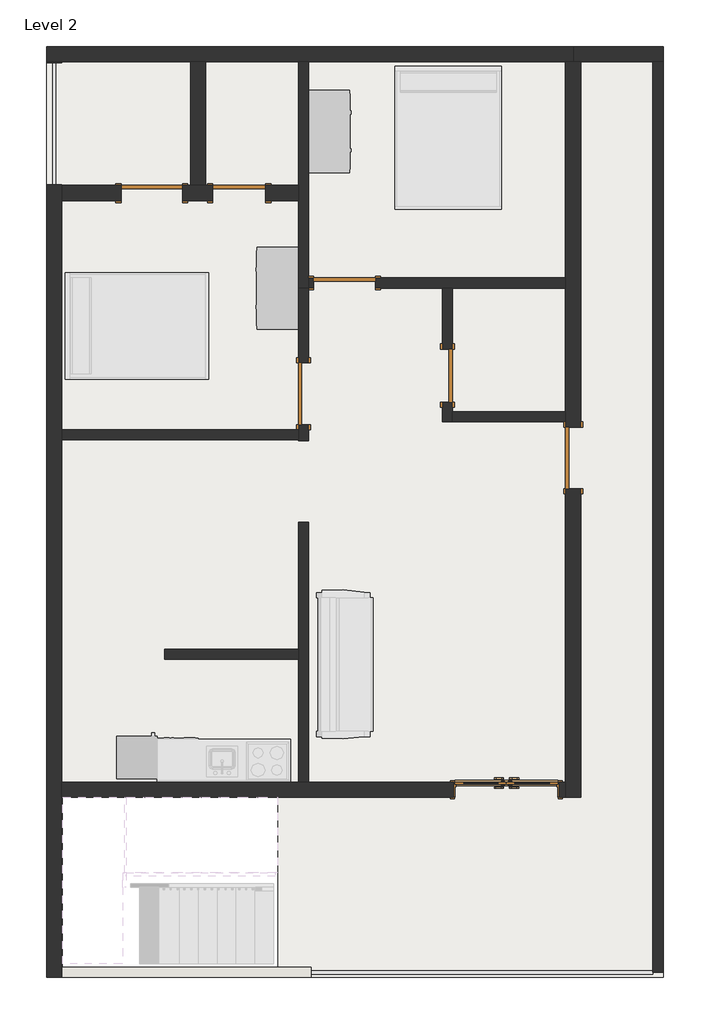
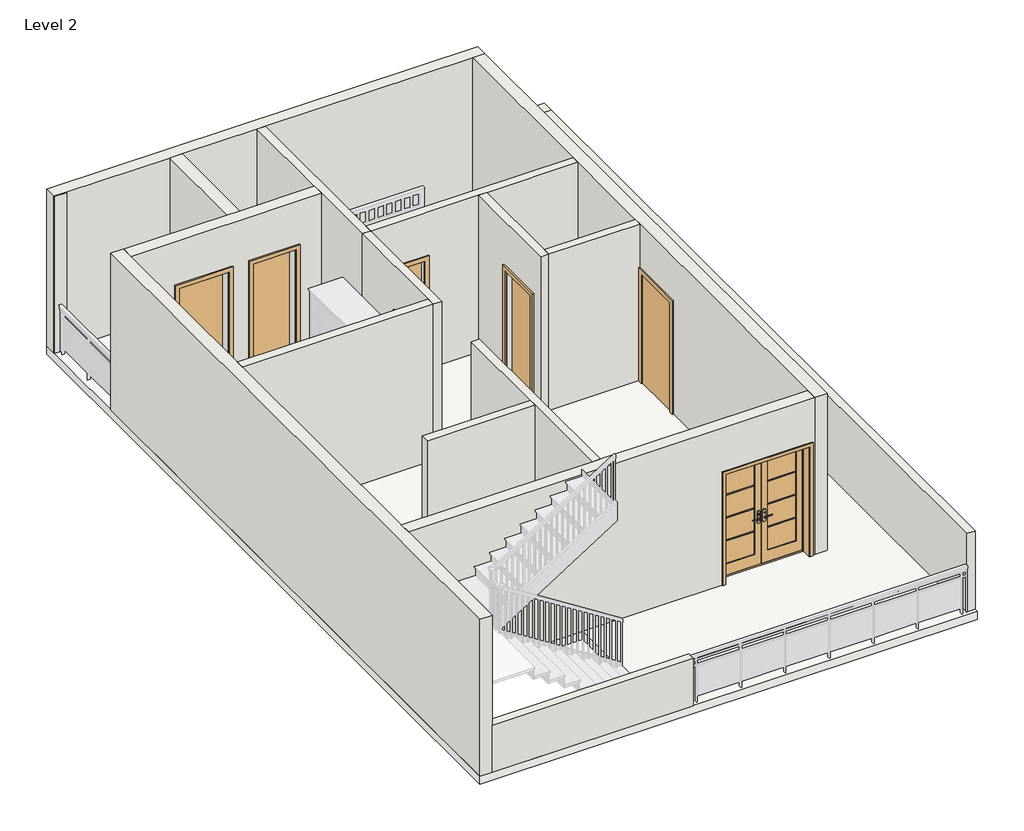
# One storey, part 1 of 2: 18 walls, 7 doors, 1 slab.
"""IFC4 building model written with IfcOpenShell, lengths in millimetres."""

from ifc_helpers import new_model, si_unit, frame, origin, place, context, project, spatial, polyline, outline, extrude, faceted_brep, transform, mapped, element, save
from components import door_014e9f54, door_486760f8, door_b804d09e, door_686f89d2, door_0ca8825f

model = new_model("IFC4")

# Units and contexts
model_context = context("Model", 3, world=origin())
ifc_project = project(units=[si_unit("LENGTHUNIT", "METRE", prefix="MILLI")], contexts=[model_context])

# Site, building, storey
site = spatial("IfcSite", under=ifc_project)
building = spatial("IfcBuilding", under=site)
storey = spatial("IfcBuildingStorey", under=building, Name="Level 2", Elevation=3200.4)

# Doors
placement = place(None, origin())
door_shape = door_014e9f54(model_context)
element("IfcDoor", 1, ObjectType="Door-Exterior-Double-Full Glass-Wood_Clad : 60\" x 84\"", at=placement, inside=storey, context=model_context, shape_type="MappedRepresentation", body=[
    mapped(door_shape, transform((-4531.8683044, -1257.1141189, 3200.4), x_axis=(1.0, 0.0, 0.0), y_axis=(0.0, 1.0, 0.0), z_axis=(0.0, 0.0, 1.0))),
])
door_2_shape = door_486760f8(model_context)
element("IfcDoor", 2, ObjectType="Single-Flush : 2'7\"", at=placement, inside=storey, context=model_context, shape_type="MappedRepresentation", body=[
    mapped(door_2_shape, transform((-8494.2683044, 7578.9108811, 3200.4), x_axis=(-1.0, 0.0, 0.0), y_axis=(0.0, -1.0, 0.0), z_axis=(0.0, 0.0, 1.0))),
])
door_3_shape = door_b804d09e(model_context)
element("IfcDoor", 3, ObjectType="Single-Flush : 2'7\"", at=placement, inside=storey, context=model_context, shape_type="MappedRepresentation", body=[
    mapped(door_3_shape, transform((-5408.1683044, 4873.8108811, 3200.4), x_axis=(0.0, -1.0, 0.0), y_axis=(1.0, 0.0, 0.0), z_axis=(0.0, 0.0, 1.0))),
])
door_4_shape = door_686f89d2(model_context)
element("IfcDoor", 4, ObjectType="Single-Flush : 36\" x 84\"", at=placement, inside=storey, context=model_context, shape_type="MappedRepresentation", body=[
    mapped(door_4_shape, transform((-6932.1683044, 6245.4108811, 3200.4), x_axis=(-1.0, 0.0, 0.0), y_axis=(0.0, -1.0, 0.0), z_axis=(0.0, 0.0, 1.0))),
])
element("IfcDoor", 5, ObjectType="Single-Flush : 36\" x 84\"", at=placement, inside=storey, context=model_context, shape_type="MappedRepresentation", body=[
    mapped(door_4_shape, transform((-7541.7683044, 4607.1108811, 3200.4), x_axis=(0.0, -1.0, 0.0), y_axis=(1.0, 0.0, 0.0), z_axis=(0.0, 0.0, 1.0))),
])
door_5_shape = door_0ca8825f(model_context)
element("IfcDoor", 6, ObjectType="Single-Flush : 36\" x 84\"", at=placement, inside=storey, context=model_context, shape_type="MappedRepresentation", body=[
    mapped(door_5_shape, transform((-9789.6683044, 7578.9108811, 3200.4), x_axis=(1.0, 0.0, 0.0), y_axis=(0.0, 1.0, 0.0), z_axis=(0.0, 0.0, 1.0))),
])
element("IfcDoor", 7, ObjectType="Single-Flush : 36\" x 84\"", at=placement, inside=storey, context=model_context, shape_type="MappedRepresentation", body=[
    mapped(door_5_shape, transform((-3541.2683044, 3654.6108811, 3200.4), x_axis=(0.0, 1.0, 0.0), y_axis=(-1.0, 0.0, 0.0), z_axis=(0.0, 0.0, 1.0))),
])

# Slab
element("IfcSlab", 8, ObjectType="6\"", at=placement, inside=storey, context=model_context, shape_type="SweptSolid", body=[
    extrude(outline(polyline([(-2207.7683044, 9750.6108811), (-2207.7683044, -4041.5891189), (-11351.7683044, -4041.5891189), (-11351.7683044, 9750.6108811), (-2207.7683044, 9750.6108811)]), holes=[polyline([(-7922.7683044, -1374.5891189), (-11110.4683044, -1374.5891189), (-11110.4683044, -3889.1891189), (-7922.7683044, -3889.1891189), (-7922.7683044, -1374.5891189)])]), frame((0.0, 0.0, 3048.0), z_axis=(0.0, 0.0, 1.0), x_axis=(1.0, 0.0, 0.0)), (0.0, 0.0, 1.0), 152.4),
])

# Walls
element("IfcWall", 9, ObjectType="6\"", at=placement, inside=storey, context=model_context, shape_type="SweptSolid", body=[
    extrude(outline(polyline([(-2360.1683044, -3965.3891189), (-2360.1683044, 9522.0108811), (-2207.7683044, 9522.0108811), (-2207.7683044, -3965.3891189), (-2360.1683044, -3965.3891189)])), frame((0.0, 0.0, 3200.4), z_axis=(0.0, 0.0, 1.0), x_axis=(1.0, 0.0, 0.0)), (0.0, 0.0, 1.0), 1524.0),
])
element("IfcWall", 10, ObjectType="6\"", at=placement, inside=storey, context=model_context, shape_type="SweptSolid", body=[
    extrude(outline(polyline([(-11123.1683044, -3889.1891189), (-7427.4683044, -3889.1891189), (-7427.4683044, -4041.5891189), (-11123.1683044, -4041.5891189), (-11123.1683044, -3889.1891189)])), frame((0.0, 0.0, 3200.4), z_axis=(0.0, 0.0, 1.0), x_axis=(1.0, 0.0, 0.0)), (0.0, 0.0, 1.0), 914.4),
])
element("IfcWall", 11, ObjectType="6\" 2", at=placement, inside=storey, context=model_context, shape_type="Brep", body=[
    faceted_brep([(-7617.9683044, 9522.0108811, 3200.4), (-7617.9683044, 7693.2108811, 3200.4), (-7617.9683044, 7464.6108811, 3200.4), (-7617.9683044, 6169.2108811, 3200.4), (-7617.9683044, 6169.2108811, 6248.4), (-7617.9683044, 7464.6108811, 6248.4), (-7617.9683044, 7693.2108811, 6248.4), (-7617.9683044, 9522.0108811, 6248.4), (-7465.5683044, 9522.0108811, 3200.4), (-7465.5683044, 9522.0108811, 6248.4), (-7465.5683044, 6321.6108811, 6248.4), (-7465.5683044, 6169.2108811, 6248.4), (-7465.5683044, 6169.2108811, 3200.4), (-7465.5683044, 6321.6108811, 3200.4)], [[[0, 1, 2, 3, 4, 5, 6, 7]], [[8, 9, 10, 11, 12, 13]], [[3, 2, 1, 0, 8, 13, 12]], [[7, 6, 5, 4, 11, 10, 9]], [[0, 7, 9, 8]], [[4, 3, 12, 11]]]),
])
element("IfcWall", 12, ObjectType="6\" 2", at=placement, inside=storey, context=model_context, shape_type="Brep", body=[
    faceted_brep([(-7465.5683044, 6169.2108811, 3200.4), (-7389.3683044, 6169.2108811, 3200.4), (-7389.3683044, 6169.2108811, 5334.0), (-6474.9683044, 6169.2108811, 5334.0), (-6474.9683044, 6169.2108811, 3200.4), (-5484.3683044, 6169.2108811, 3200.4), (-5331.9683044, 6169.2108811, 3200.4), (-3655.5683044, 6169.2108811, 3200.4), (-3655.5683044, 6169.2108811, 6248.4), (-5331.9683044, 6169.2108811, 6248.4), (-5484.3683044, 6169.2108811, 6248.4), (-7465.5683044, 6169.2108811, 6248.4), (-7389.3683044, 6321.6108811, 5334.0), (-7389.3683044, 6321.6108811, 3200.4), (-7465.5683044, 6321.6108811, 3200.4), (-7465.5683044, 6321.6108811, 6248.4), (-3655.5683044, 6321.6108811, 6248.4), (-3655.5683044, 6321.6108811, 3200.4), (-6474.9683044, 6321.6108811, 3200.4), (-6474.9683044, 6321.6108811, 5334.0)], [[[0, 1, 2, 3, 4, 5, 6, 7, 8, 9, 10, 11]], [[12, 13, 14, 15, 16, 17, 18, 19]], [[18, 17, 7, 6, 5, 4]], [[14, 13, 1, 0]], [[11, 10, 9, 8, 16, 15]], [[0, 11, 15, 14]], [[8, 7, 17, 16]], [[2, 1, 13, 12]], [[3, 2, 12, 19]], [[4, 3, 19, 18]]]),
])
element("IfcWall", 13, ObjectType="6\" 2", at=placement, inside=storey, context=model_context, shape_type="Brep", body=[
    faceted_brep([(-7617.9683044, 4149.9108811, 5334.0), (-7617.9683044, 4149.9108811, 3200.4), (-7617.9683044, 4073.7108811, 3200.4), (-7617.9683044, 3921.3108811, 3200.4), (-7617.9683044, 3908.6108811, 3200.4), (-7617.9683044, 3908.6108811, 6248.4), (-7617.9683044, 3921.3108811, 6248.4), (-7617.9683044, 4073.7108811, 6248.4), (-7617.9683044, 6169.2108811, 6248.4), (-7617.9683044, 6169.2108811, 3200.4), (-7617.9683044, 5064.3108811, 3200.4), (-7617.9683044, 5064.3108811, 5334.0), (-7465.5683044, 3908.6108811, 3200.4), (-7465.5683044, 4149.9108811, 3200.4), (-7465.5683044, 4149.9108811, 5334.0), (-7465.5683044, 5064.3108811, 5334.0), (-7465.5683044, 5064.3108811, 3200.4), (-7465.5683044, 6169.2108811, 3200.4), (-7465.5683044, 6169.2108811, 6248.4), (-7465.5683044, 3908.6108811, 6248.4)], [[[0, 1, 2, 3, 4, 5, 6, 7, 8, 9, 10, 11]], [[12, 13, 14, 15, 16, 17, 18, 19]], [[10, 9, 17, 16]], [[4, 3, 2, 1, 13, 12]], [[5, 4, 12, 19]], [[8, 7, 6, 5, 19, 18]], [[9, 8, 18, 17]], [[14, 13, 1, 0]], [[15, 14, 0, 11]], [[16, 15, 11, 10]]]),
])
element("IfcWall", 14, ObjectType="6\" 2", at=placement, inside=storey, context=model_context, shape_type="SweptSolid", body=[
    extrude(outline(polyline([(-7617.9683044, 3921.3108811), (-11123.1683044, 3921.3108811), (-11123.1683044, 4073.7108811), (-7617.9683044, 4073.7108811), (-7617.9683044, 3921.3108811)])), frame((0.0, 0.0, 3200.4), z_axis=(0.0, 0.0, 1.0), x_axis=(1.0, 0.0, 0.0)), (0.0, 0.0, 1.0), 3048.0),
])
element("IfcWall", 15, ObjectType="6\" 2", at=placement, inside=storey, context=model_context, shape_type="SweptSolid", body=[
    extrude(outline(polyline([(-9599.1683044, 822.5108811), (-7617.9683044, 822.5108811), (-7617.9683044, 670.1108811), (-9599.1683044, 670.1108811), (-9599.1683044, 822.5108811)])), frame((0.0, 0.0, 3200.4), z_axis=(0.0, 0.0, 1.0), x_axis=(1.0, 0.0, 0.0)), (0.0, 0.0, 1.0), 3048.0),
])
element("IfcWall", 16, ObjectType="6\" 2", at=placement, inside=storey, context=model_context, shape_type="Brep", body=[
    faceted_brep([(-5484.3683044, 4480.1108811, 5334.0), (-5484.3683044, 4480.1108811, 3200.4), (-5484.3683044, 4188.0108811, 3200.4), (-5484.3683044, 4188.0108811, 6248.4), (-5484.3683044, 6169.2108811, 6248.4), (-5484.3683044, 6169.2108811, 3200.4), (-5484.3683044, 5267.5108811, 3200.4), (-5484.3683044, 5267.5108811, 5334.0), (-5331.9683044, 4188.0108811, 3200.4), (-5331.9683044, 4480.1108811, 3200.4), (-5331.9683044, 4480.1108811, 5334.0), (-5331.9683044, 5267.5108811, 5334.0), (-5331.9683044, 5267.5108811, 3200.4), (-5331.9683044, 6169.2108811, 3200.4), (-5331.9683044, 6169.2108811, 6248.4), (-5331.9683044, 4340.4108811, 6248.4), (-5331.9683044, 4188.0108811, 6248.4), (-5331.9683044, 4188.0108811, 3214.2133607)], [[[0, 1, 2, 3, 4, 5, 6, 7]], [[8, 9, 10, 11, 12, 13, 14, 15, 16, 17]], [[6, 5, 13, 12]], [[2, 1, 9, 8]], [[4, 3, 16, 15, 14]], [[5, 4, 14, 13]], [[3, 2, 8, 17, 16]], [[10, 9, 1, 0]], [[11, 10, 0, 7]], [[12, 11, 7, 6]]]),
])
element("IfcWall", 17, ObjectType="6\" 2", at=placement, inside=storey, context=model_context, shape_type="SweptSolid", body=[
    extrude(outline(polyline([(-3655.5683044, 4188.0108811), (-5331.9683044, 4188.0108811), (-5331.9683044, 4340.4108811), (-3655.5683044, 4340.4108811), (-3655.5683044, 4188.0108811)])), frame((0.0, 0.0, 3214.2133607), z_axis=(0.0, 0.0, 1.0), x_axis=(1.0, 0.0, 0.0)), (0.0, 0.0, 1.0), 3034.1866393),
])
element("IfcWall", 18, ObjectType="6\" 2", at=placement, inside=storey, context=model_context, shape_type="Brep", body=[
    faceted_brep([(-7617.9683044, 2702.1108811, 3200.4), (-7617.9683044, 822.5108811, 3200.4), (-7617.9683044, 670.1108811, 3200.4), (-7617.9683044, -1145.9891189, 3200.4), (-7617.9683044, -1145.9891189, 6248.4), (-7617.9683044, 670.1108811, 6248.4), (-7617.9683044, 822.5108811, 6248.4), (-7617.9683044, 2702.1108811, 6248.4), (-7465.5683044, 2702.1108811, 3200.4), (-7465.5683044, 2702.1108811, 6248.4), (-7465.5683044, -1145.9891189, 6248.4), (-7465.5683044, -1145.9891189, 3200.4)], [[[0, 1, 2, 3, 4, 5, 6, 7]], [[8, 9, 10, 11]], [[3, 2, 1, 0, 8, 11]], [[7, 6, 5, 4, 10, 9]], [[0, 7, 9, 8]], [[4, 3, 11, 10]]]),
])
element("IfcWall", 19, ObjectType="9\"", at=placement, inside=storey, context=model_context, shape_type="Brep", body=[
    faceted_brep([(-11351.7683044, 9522.0108811, 3200.4), (-11123.1683044, 9522.0108811, 3200.4), (-9218.1683044, 9522.0108811, 3200.4), (-8989.5683044, 9522.0108811, 3200.4), (-7617.9683044, 9522.0108811, 3200.4), (-7465.5683044, 9522.0108811, 3200.4), (-3655.5683044, 9522.0108811, 3200.4), (-3541.2683044, 9522.0108811, 3200.4), (-3541.2683044, 9522.0108811, 4724.4), (-3426.9683044, 9522.0108811, 4724.4), (-3426.9683044, 9522.0108811, 6248.4), (-3655.5683044, 9522.0108811, 6248.4), (-7465.5683044, 9522.0108811, 6248.4), (-7617.9683044, 9522.0108811, 6248.4), (-8989.5683044, 9522.0108811, 6248.4), (-9218.1683044, 9522.0108811, 6248.4), (-11123.1683044, 9522.0108811, 6248.4), (-11351.7683044, 9522.0108811, 6248.4), (-11351.7683044, 9750.6108811, 3200.4), (-11351.7683044, 9750.6108811, 6248.4), (-3426.9683044, 9750.6108811, 6248.4), (-3426.9683044, 9750.6108811, 4724.4), (-3541.2683044, 9750.6108811, 4724.4), (-3541.2683044, 9750.6108811, 3200.4)], [[[0, 1, 2, 3, 4, 5, 6, 7, 8, 9, 10, 11, 12, 13, 14, 15, 16, 17]], [[18, 19, 20, 21, 22, 23]], [[7, 6, 5, 4, 3, 2, 1, 0, 18, 23]], [[17, 16, 15, 14, 13, 12, 11, 10, 20, 19]], [[0, 17, 19, 18]], [[8, 7, 23, 22]], [[21, 9, 8, 22]], [[10, 9, 21, 20]]]),
])
element("IfcWall", 20, ObjectType="9\"", at=placement, inside=storey, context=model_context, shape_type="Brep", body=[
    faceted_brep([(-11123.1683044, -4041.5891189, 3200.4), (-11123.1683044, -3889.1891189, 3200.4), (-11123.1683044, -1374.5891189, 3200.4), (-11123.1683044, -1145.9891189, 3200.4), (-11123.1683044, 3921.3108811, 3200.4), (-11123.1683044, 4073.7108811, 3200.4), (-11123.1683044, 7464.6108811, 3200.4), (-11123.1683044, 7693.2108811, 3200.4), (-11123.1683044, 7705.9108811, 3200.4), (-11123.1683044, 7705.9108811, 6248.4), (-11123.1683044, 7693.2108811, 6248.4), (-11123.1683044, 7464.6108811, 6248.4), (-11123.1683044, 4073.7108811, 6248.4), (-11123.1683044, 3921.3108811, 6248.4), (-11123.1683044, -1145.9891189, 6248.4), (-11123.1683044, -1374.5891189, 6248.4), (-11123.1683044, -4041.5891189, 6248.4), (-11123.1683044, -4041.5891189, 4114.8), (-11351.7683044, -4041.5891189, 3200.4), (-11351.7683044, -4041.5891189, 6248.4), (-11351.7683044, 7705.9108811, 6248.4), (-11351.7683044, 7705.9108811, 3200.4)], [[[0, 1, 2, 3, 4, 5, 6, 7, 8, 9, 10, 11, 12, 13, 14, 15, 16, 17]], [[18, 19, 20, 21]], [[8, 7, 6, 5, 4, 3, 2, 1, 0, 18, 21]], [[9, 8, 21, 20]], [[16, 15, 14, 13, 12, 11, 10, 9, 20, 19]], [[0, 17, 16, 19, 18]]]),
])
element("IfcWall", 21, ObjectType="9\"", at=placement, inside=storey, context=model_context, shape_type="Brep", body=[
    faceted_brep([(-3655.5683044, 9522.0108811, 3200.4), (-3655.5683044, 6321.6108811, 3200.4), (-3655.5683044, 6169.2108811, 3200.4), (-3655.5683044, 4111.8108811, 3200.4), (-3655.5683044, 4111.8108811, 5334.0), (-3655.5683044, 3197.4108811, 5334.0), (-3655.5683044, 3197.4108811, 3200.4), (-3655.5683044, -1145.9891189, 3200.4), (-3655.5683044, -1374.5891189, 3200.4), (-3655.5683044, -1374.5891189, 6248.4), (-3655.5683044, -1145.9891189, 6248.4), (-3655.5683044, 4188.0108811, 6248.4), (-3655.5683044, 4340.4108811, 6248.4), (-3655.5683044, 6169.2108811, 6248.4), (-3655.5683044, 6321.6108811, 6248.4), (-3655.5683044, 9522.0108811, 6248.4), (-3426.9683044, 4111.8108811, 5334.0), (-3426.9683044, 4111.8108811, 3200.4), (-3426.9683044, 9522.0108811, 3200.4), (-3426.9683044, 9522.0108811, 4724.4), (-3426.9683044, 9522.0108811, 6248.4), (-3426.9683044, -1374.5891189, 6248.4), (-3426.9683044, -1374.5891189, 3200.4), (-3426.9683044, 3197.4108811, 3200.4), (-3426.9683044, 3197.4108811, 5334.0), (-3541.2683044, 9522.0108811, 3200.4)], [[[0, 1, 2, 3, 4, 5, 6, 7, 8, 9, 10, 11, 12, 13, 14, 15]], [[16, 17, 18, 19, 20, 21, 22, 23, 24]], [[23, 22, 8, 7, 6]], [[18, 17, 3, 2, 1, 0, 25]], [[15, 14, 13, 12, 11, 10, 9, 21, 20]], [[9, 8, 22, 21]], [[15, 20, 19, 18, 25, 0]], [[4, 3, 17, 16]], [[5, 4, 16, 24]], [[6, 5, 24, 23]]]),
])
element("IfcWall", 22, ObjectType="9\"", at=placement, inside=storey, context=model_context, shape_type="Brep", body=[
    faceted_brep([(-11123.1683044, -1145.9891189, 6248.4), (-7617.9683044, -1145.9891189, 6248.4), (-7465.5683044, -1145.9891189, 6248.4), (-3655.5683044, -1145.9891189, 6248.4), (-3655.5683044, -1145.9891189, 3200.4), (-3744.4683044, -1145.9891189, 3200.4), (-3744.4683044, -1145.9891189, 5359.4), (-5319.2683044, -1145.9891189, 5359.4), (-5319.2683044, -1145.9891189, 3200.4), (-7465.5683044, -1145.9891189, 3200.4), (-7617.9683044, -1145.9891189, 3200.4), (-11123.1683044, -1145.9891189, 3200.4), (-3655.5683044, -1374.5891189, 6248.4), (-11123.1683044, -1374.5891189, 6248.4), (-11123.1683044, -1374.5891189, 3200.4), (-5319.2683044, -1374.5891189, 3200.4), (-5319.2683044, -1374.5891189, 5359.4), (-3744.4683044, -1374.5891189, 5359.4), (-3744.4683044, -1374.5891189, 3200.4), (-3655.5683044, -1374.5891189, 3200.4)], [[[0, 1, 2, 3, 4, 5, 6, 7, 8, 9, 10, 11]], [[12, 13, 14, 15, 16, 17, 18, 19]], [[4, 19, 18, 5]], [[14, 11, 10, 9, 8, 15]], [[3, 2, 1, 0, 13, 12]], [[4, 3, 12, 19]], [[0, 11, 14, 13]], [[17, 6, 5, 18]], [[6, 17, 16, 7]], [[7, 16, 15, 8]]]),
])
element("IfcWall", 23, ObjectType="9\"", at=placement, inside=storey, context=model_context, shape_type="Brep", body=[
    faceted_brep([(-9332.4683044, 7464.6108811, 3200.4), (-8887.9683044, 7464.6108811, 3200.4), (-8887.9683044, 7464.6108811, 5334.0), (-8100.5683044, 7464.6108811, 5334.0), (-8100.5683044, 7464.6108811, 3200.4), (-7617.9683044, 7464.6108811, 3200.4), (-7617.9683044, 7464.6108811, 6248.4), (-11123.1683044, 7464.6108811, 6248.4), (-11123.1683044, 7464.6108811, 3200.4), (-10246.8683044, 7464.6108811, 3200.4), (-10246.8683044, 7464.6108811, 5334.0), (-9332.4683044, 7464.6108811, 5334.0), (-8887.9683044, 7693.2108811, 5334.0), (-8887.9683044, 7693.2108811, 3200.4), (-8989.5683044, 7693.2108811, 3200.4), (-9218.1683044, 7693.2108811, 3200.4), (-9332.4683044, 7693.2108811, 3200.4), (-9332.4683044, 7693.2108811, 5334.0), (-10246.8683044, 7693.2108811, 5334.0), (-10246.8683044, 7693.2108811, 3200.4), (-11123.1683044, 7693.2108811, 3200.4), (-11123.1683044, 7693.2108811, 6248.4), (-9218.1683044, 7693.2108811, 6248.4), (-8989.5683044, 7693.2108811, 6248.4), (-7617.9683044, 7693.2108811, 6248.4), (-7617.9683044, 7693.2108811, 3200.4), (-8100.5683044, 7693.2108811, 3200.4), (-8100.5683044, 7693.2108811, 5334.0)], [[[0, 1, 2, 3, 4, 5, 6, 7, 8, 9, 10, 11]], [[12, 13, 14, 15, 16, 17, 18, 19, 20, 21, 22, 23, 24, 25, 26, 27]], [[9, 8, 20, 19]], [[26, 25, 5, 4]], [[16, 15, 14, 13, 1, 0]], [[7, 6, 24, 23, 22, 21]], [[8, 7, 21, 20]], [[6, 5, 25, 24]], [[17, 16, 0, 11]], [[18, 17, 11, 10]], [[19, 18, 10, 9]], [[2, 1, 13, 12]], [[3, 2, 12, 27]], [[4, 3, 27, 26]]]),
])
element("IfcWall", 24, ObjectType="9\"", at=placement, inside=storey, context=model_context, shape_type="SweptSolid", body=[
    extrude(outline(polyline([(-8989.5683044, 9522.0108811), (-8989.5683044, 7693.2108811), (-9218.1683044, 7693.2108811), (-9218.1683044, 9522.0108811), (-8989.5683044, 9522.0108811)])), frame((0.0, 0.0, 3200.4), z_axis=(0.0, 0.0, 1.0), x_axis=(1.0, 0.0, 0.0)), (0.0, 0.0, 1.0), 3048.0),
])
element("IfcWall", 25, ObjectType="9\"", at=placement, inside=storey, context=model_context, shape_type="Brep", body=[
    faceted_brep([(-3541.2683044, 9522.0108811, 3200.4), (-3426.9683044, 9522.0108811, 3200.4), (-2360.1683044, 9522.0108811, 3200.4), (-2207.7683044, 9522.0108811, 3200.4), (-2207.7683044, 9522.0108811, 4724.4), (-2360.1683044, 9522.0108811, 4724.4), (-3426.9683044, 9522.0108811, 4724.4), (-3541.2683044, 9522.0108811, 4724.4), (-3541.2683044, 9750.6108811, 3200.4), (-3541.2683044, 9750.6108811, 4724.4), (-3426.9683044, 9750.6108811, 4724.4), (-2207.7683044, 9750.6108811, 4724.4), (-2207.7683044, 9750.6108811, 3200.4)], [[[0, 1, 2, 3, 4, 5, 6, 7]], [[8, 9, 10, 11, 12]], [[3, 2, 1, 0, 8, 12]], [[7, 6, 5, 4, 11, 10, 9]], [[0, 7, 9, 8]], [[4, 3, 12, 11]]]),
])
element("IfcWall", 26, ObjectType="9\"", at=placement, inside=storey, context=model_context, shape_type="SweptSolid", body=[
    extrude(outline(polyline([(-11123.1683044, 9522.0108811), (-11123.1683044, 9509.3108811), (-11351.7683044, 9509.3108811), (-11351.7683044, 9522.0108811), (-11123.1683044, 9522.0108811)])), frame((0.0, 0.0, 3200.4), z_axis=(0.0, 0.0, 1.0), x_axis=(1.0, 0.0, 0.0)), (0.0, 0.0, 1.0), 3048.0),
])

save(model, "model.ifc")

# Revit data of these elements
# Type "Door-Exterior-Double-Full Glass-Wood_Clad : 60\" x 84\""
#   Type Mark = "9"
#   Assembly Code = "B2030100"
#   Analytic Construction = "French door, wood frame with double glass"
#   Top Rail = 0' - 4 11/16"
#   Threshold Offset [instance default] = 0' - 0 1/2"
#   Thickness = 0' - 1 3/8"
#   Thermal Resistance (R) = 1.9158 (h·ft²·°F)/BTU
#   Swing Angle [instance default] = 90.00°
#   Stiles = 0' - 4 3/4"
#   Rough Width = 5' - 2"
#   Rough Height = 7' - 1"
#   Panel Width = 2' - 6"
#   Door Offset [instance default] = 0' - 0"
#   Height = 7' - 0"
#   Width = 5' - 0"
#   Heat Transfer Coefficient (U) = 0.5220 BTU/(h·ft²·°F)
#   Bottom Rail = 0' - 9 1/8"
#   Exterior Trim [instance default] = yes
#   Threshold [instance default] = yes
#   Show Grill [instance default] = yes
#   Function = 1
#   Trim Material = Cherry
#   Threshold Material = Cherry
#   Panel Material = Cherry
#   Glazing = Glass
#   Frame Material = Cherry
#   Door Handle Material = Aluminum
#   Visual Light Transmittance = 0
#   Solar Heat Gain Coefficient = 0
#   Wall Closure = (empty or 0)
#   Construction Type = (empty or 0)
# Type "Single-Flush : 2'7\""
#   Type Mark = "8"
#   Construction Type Id = "MDOOR"
#   Assembly Code = "C1020"
#   Analytic Construction = "Metal"
#   Thickness = 0' - 2"
#   Heat Transfer Coefficient (U) = 0.651978 BTU/(h·ft²·°F)
#   Height = 7' - 0"
#   Trim Projection Ext = 0' - 1"
#   Trim Projection Int = 0' - 1"
#   Trim Width = 0' - 3"
#   Width = 2' - 7"
#   Define Thermal Properties by = 1
#   Door Material = Door - Panel
#   Frame Material = Door - Frame
#   Visual Light Transmittance = 0
#   Solar Heat Gain Coefficient = 0
#   Function = (empty or 0)
#   Wall Closure = (empty or 0)
# Type "Single-Flush : 36\" x 84\""
#   Type Mark = "1"
#   Construction Type Id = "MDOOR"
#   Assembly Code = "C1020"
#   Analytic Construction = "Metal"
#   Thickness = 0' - 2"
#   Heat Transfer Coefficient (U) = 0.651978 BTU/(h·ft²·°F)
#   Height = 7' - 0"
#   Trim Projection Ext = 0' - 1"
#   Trim Projection Int = 0' - 1"
#   Trim Width = 0' - 3"
#   Width = 3' - 0"
#   Define Thermal Properties by = 1
#   Door Material = Door - Panel
#   Frame Material = Door - Frame
#   Visual Light Transmittance = 0
#   Solar Heat Gain Coefficient = 0
#   Function = (empty or 0)
#   Wall Closure = (empty or 0)
# Type "6\""
#   Assembly Code = "B1010"
#   Function = 0
#   Layers, outside or top first: 0' - 6" "floor" (function 1)
# Type "6\""
#   Assembly Code = "B2010"
#   Layers, outside or top first: 0' - 6" "ext wall" (function 1)
# Type "6\" 2"
#   Assembly Code = "B2010"
#   Layers, outside or top first: 0' - 6" no material (function 1)
# Type "9\""
#   Assembly Code = "B2010"
#   Layers, outside or top first: 0' - 9" "ext wall" (function 1)
# Element 1 (IfcDoor, "Door-Exterior-Double-Full Glass-Wood_Clad : 60\" x 84\"")
#   Threshold Offset = 0' - 0 1/2"
#   Swing Angle = 90.00°
#   Door Offset = 0' - 0"
#   Threshold = yes
#   Show Grill = yes
#   Exterior Trim = yes
#   Phase Created = New Construction
#   Materials on its faces: "Cherry", "Aluminum", "Glass"
# Elements 2, 3 (IfcDoor, "Single-Flush : 2'7\"")
#   Phase Created = New Construction
#   Materials on its faces: "Door - Frame", "Door - Panel"
# Elements 4, 5, 6, 7 (IfcDoor, "Single-Flush : 36\" x 84\"")
#   Phase Created = New Construction
#   Materials on its faces: "Door - Frame", "Door - Panel"
# Element 8 (IfcSlab, "6\"")
#   Height Offset From Level = 0' - 0"
#   Phase Created = New Construction
#   Materials on its faces: "floor"
# Element 9 (IfcWall, "6\"")
#   Top Offset = 0' - 0"
#   Base Offset = 0' - 0"
#   Unconnected Height = 5' - 0"
#   wall height = 5' - 0"
#   Phase Created = New Construction
#   Base Constraint = Level 2
#   Materials on its faces: "ext wall"
# Element 10 (IfcWall, "6\"")
#   Top Offset = 0' - 0"
#   Base Offset = 0' - 0"
#   Unconnected Height = 3' - 0"
#   wall height = 3' - 0"
#   Phase Created = New Construction
#   Base Constraint = Level 2
#   Materials on its faces: "ext wall"
# Elements 11, 12, 13, 14, 15, 16, 18 (IfcWall, "6\" 2")
#   Top Offset = 0' - 0"
#   Base Offset = 0' - 0"
#   Unconnected Height = 10' - 0"
#   wall height = 10' - 0"
#   Phase Created = New Construction
#   Base Constraint = Level 2
#   Materials on its faces: "Default Wall"
# Element 17 (IfcWall, "6\" 2")
#   built-in parameter 1001111 = 0' - 0.54383"
#   Top Offset = 0' - 0"
#   Base Offset = 0' - 0.54383"
#   Unconnected Height = 9' - 11.45617"
#   wall height = 9' - 11.45617"
#   Phase Created = New Construction
#   Base Constraint = Level 2
#   Materials on its faces: "Default Wall"
# Elements 19, 20, 21, 22, 23, 24, 26 (IfcWall, "9\"")
#   Top Offset = 0' - 0"
#   Base Offset = 0' - 0"
#   Unconnected Height = 10' - 0"
#   wall height = 10' - 0"
#   Phase Created = New Construction
#   Base Constraint = Level 2
#   Materials on its faces: "ext wall"
# Element 25 (IfcWall, "9\"")
#   Top Offset = 0' - 0"
#   Base Offset = 0' - 0"
#   Unconnected Height = 5' - 0"
#   wall height = 5' - 0"
#   Phase Created = New Construction
#   Base Constraint = Level 2
#   Materials on its faces: "ext wall"
# Materials
#   "Cherry": class "Wood", colour RGB 226 177 128, transparency 0, Description = "Prunus Serotina", Cost = 0
#   "Glass": class "Glass", colour RGB 0 128 192, transparency 0.75, Description = "Soda Lime Glass", Cost = 0
#   "Aluminum": class "Metal", colour RGB 247 247 247, transparency 0, Description = "Aluminum 6061", Cost = 0
#   "Door - Panel": class "Wood", colour RGB 210 159 95, transparency 0
#   "Door - Frame": colour RGB 118 70 51, transparency 0
#   "floor": class "Generic", colour RGB 146 137 125, transparency 0, Cost = 0
#   "ext wall": class "Generic", colour RGB 230 213 172, transparency 0, Cost = 0
#   "Default Wall": colour RGB 128 128 128, transparency 0
